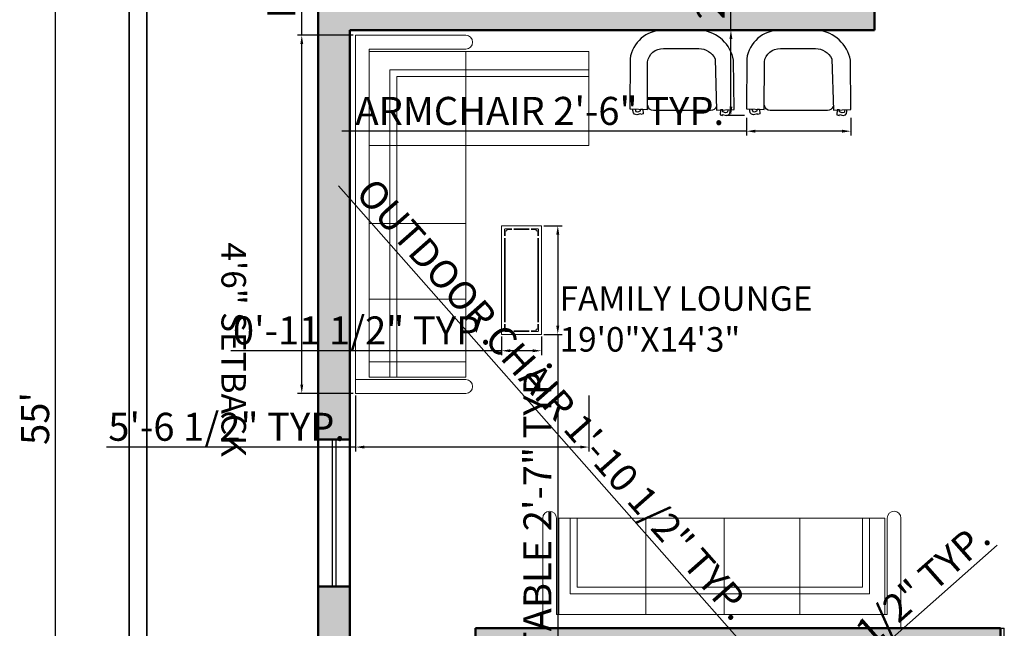
# Model space of a CAD drawing. Units: inches. Extents: x 3008 to 4088, y 1255 to 2137.
# Tile 25 of 30: x 3572 to 3853, y 1620 to 1794. Entities that reach past the tile are written whole.
import ezdxf

# ---------------------------------------------------------------- set-up
doc = ezdxf.new("R2010")
doc.units = ezdxf.units.IN
doc.layers.add('2D', color=7, linetype='Continuous')
for name, color, linetype, lineweight in [('A-ANNO-DIMS', 2, 'Continuous', 18), ('A-ANNO-TEXT', 7, 'Continuous', 18), ('A-AREA-IDEN', 7, 'Continuous', 18), ('A-DOOR', 4, 'Continuous', 25), ('A-FURN', 8, 'Continuous', 18), ('A-GLAZ', 4, 'Continuous', 25), ('A-WALL', 7, 'Continuous', 50), ('A-WALL-PATT', 8, 'Continuous', 13), ('C-PROP', 1, 'Continuous', 35)]:
    doc.layers.add(name, color=color, linetype=linetype, lineweight=lineweight)
doc.styles.get("Standard").update_dxf_attribs({"font": 'arial.ttf'})
doc.dimstyles.new('ISO-25', dxfattribs={"dimtxt": 8, "dimasz": 2.5, "dimexe": 1.25, "dimexo": 0.625, "dimtad": 1, "dimdec": 1, "dimlunit": 3, "dimtxsty": 'Standard', "dimcen": 2.5, "dimadec": 0, "dimazin": 0, "dimtfac": 1, "dimtdec": 1, "dimtmove": 0, "dimatfit": 3, "dimfxl": 1, "dimarcsym": 0})

# ---------------------------------------------------------------- blocks, each defined once
blk = doc.blocks.new('*D32')
at = {"layer": 'A-ANNO-DIMS', "color": 0, "lineweight": -2, "transparency": 16777216}
for p, q in [((3602.32, 2009.72), (3580.54, 2009.72)), ((3581.79, 2007.22), (3581.79, 1352.22)), ((3602.32, 1349.72), (3580.54, 1349.72))]:
    blk.add_line(p, q, dxfattribs=at)
at = {"layer": 'A-ANNO-DIMS', "color": 0, "transparency": 16777216}
for points in [[(3581.37, 2007.22), (3582.2, 2007.22), (3581.79, 2009.72)], [(3581.37, 1352.22), (3582.2, 1352.22), (3581.79, 1349.72)]]:
    blk.add_solid(points, dxfattribs=at)
at = {"layer": 'Defpoints', "color": 0, "transparency": 16777216}
for p in [(3602.94, 2009.72), (3581.79, 1349.72), (3602.94, 1349.72)]:
    blk.add_point(p, dxfattribs=at)
at = {"layer": 'A-ANNO-DIMS', "color": 0, "transparency": 16777216, "insert": (3577.09, 1679.72), "char_height": 8, "attachment_point": 5, "rotation": 90}
blk.add_mtext("55'", dxfattribs=at)
blk = doc.blocks.new('D1')
for p, q in [((1805.96, 1500.36), (1805.96, 1464.36)), ((1806.96, 1500.36), (1806.96, 1464.36)), ((1805.96, 1464.36), (1806.96, 1464.36))]:
    blk.add_line(p, q)
blk.add_arc((1805.96, 1464.36), 36, 0, 90)
blk = doc.blocks.new('S 1')
at = {"layer": '2D'}
blk.add_lwpolyline([(4300.17, 1811.07), (4294.36, 1811.27), (4294.5, 1827.76, -0.326306), (4305.18, 1837.77), (4318.07, 1837.77, -0.372891), (4329.09, 1828.23), (4329.16, 1811.54), (4323.28, 1811.34), (4323.21, 1827.16, 0.399039), (4317.87, 1831.63), (4306.12, 1831.63, 0.288471), (4300.71, 1828.23)], format="xyb", close=True, dxfattribs=at)
for points in [[(4296.37, 1811.14), (4296.63, 1810.34), (4297.23, 1810.21), (4298.1, 1810.54), (4298.1, 1811.14), (4298.9, 1811.14), (4299.04, 1809.54), (4298.24, 1809.34), (4298.17, 1809.61), (4296.9, 1809.27), (4296.17, 1809.47), (4295.77, 1809.94), (4295.63, 1810.74), (4295.63, 1811.21)], [(4327.35, 1811.41), (4327.09, 1810.61), (4326.49, 1810.47), (4325.62, 1810.81), (4325.62, 1811.41), (4324.82, 1811.41), (4324.68, 1809.81), (4325.48, 1809.61), (4325.55, 1809.87), (4326.82, 1809.54), (4327.55, 1809.74), (4327.95, 1810.21), (4328.09, 1811.01), (4328.09, 1811.47)]]:
    blk.add_lwpolyline(points, dxfattribs=at)
blk.add_lwpolyline([(4300.24, 1812.34, 0.33845), (4302.18, 1810.94), (4321.28, 1810.94, 0.381322), (4323.15, 1812.61, -0.892406)], format="xyb", dxfattribs=at)
blk = doc.blocks.new('TABLE-30A')
at = {"color": 0, "linetype": 'ByBlock'}
for p, q in [((0, 0), (0, 0.55)), ((0, 0.55), (1.5, 0.55)), ((1.5, 0.55), (1.5, 0)), ((0.051, 0.508), (0.042, 0.499)), ((0.042, 0.499), (0.042, 0.478)), ((0.042, 0.478), (0.072, 0.478)), ((0.042, 0.478), (0.042, 0.41)), ((0.072, 0.508), (0.051, 0.508)), ((0.051, 0.478), (0.051, 0.41)), ((0.072, 0.478), (0.072, 0.508)), ((0.072, 0.508), (0.14, 0.508)), ((0.072, 0.499), (0.14, 0.499)), ((1.331, 0.508), (0.169, 0.508)), ((1.331, 0.499), (0.169, 0.499)), ((1.428, 0.508), (1.36, 0.508)), ((1.428, 0.499), (1.36, 0.499)), ((1.428, 0.508), (1.428, 0.478)), ((1.449, 0.508), (1.428, 0.508)), ((1.428, 0.478), (1.458, 0.478)), ((1.458, 0.499), (1.449, 0.508)), ((1.449, 0.478), (1.449, 0.41)), ((1.458, 0.478), (1.458, 0.499)), ((1.458, 0.478), (1.458, 0.41)), ((0.042, 0.169), (0.042, 0.381)), ((0.051, 0.169), (0.051, 0.381)), ((1.449, 0.381), (1.449, 0.169)), ((1.458, 0.381), (1.458, 0.169)), ((0.042, 0.072), (0.042, 0.14)), ((0.051, 0.072), (0.051, 0.14)), ((1.449, 0.072), (1.449, 0.14)), ((1.458, 0.072), (1.458, 0.14)), ((1.5, 0), (0, 0)), ((0.042, 0.072), (0.042, 0.051)), ((0.072, 0.072), (0.042, 0.072)), ((0.042, 0.051), (0.051, 0.042)), ((0.051, 0.042), (0.072, 0.042)), ((0.072, 0.042), (0.072, 0.072)), ((0.072, 0.051), (0.14, 0.051)), ((0.072, 0.042), (0.14, 0.042)), ((0.169, 0.051), (1.331, 0.051)), ((0.169, 0.042), (1.331, 0.042)), ((1.428, 0.051), (1.36, 0.051)), ((1.428, 0.042), (1.36, 0.042)), ((1.428, 0.072), (1.428, 0.042)), ((1.458, 0.072), (1.428, 0.072)), ((1.428, 0.042), (1.449, 0.042)), ((1.449, 0.042), (1.458, 0.051)), ((1.458, 0.051), (1.458, 0.072))]:
    blk.add_line(p, q, dxfattribs=at)
blk = doc.blocks.new('SOFA-L')
for p, q in [((35.53, 102.74), (67.02, 102.74)), ((67.02, 102.74), (67.02, 0.37)), ((35.53, 98.8), (63.09, 98.8)), ((63.09, 98.8), (63.09, 4.97)), ((0.3, 98.14), (0.3, 71.24)), ((63.09, 98.14), (0.3, 98.14)), ((35.53, 4.97), (35.53, 98.14)), ((0.3, 92.9), (57.18, 92.9)), ((57.18, 92.9), (57.18, 4.97)), ((0.3, 90.93), (55.21, 90.93)), ((55.21, 90.93), (55.21, 4.97)), ((63.09, 71.24), (0.3, 71.24)), ((40.78, 71.24), (0.3, 71.24)), ((63.09, 48.93), (35.53, 48.93)), ((63.09, 27.28), (35.53, 27.28)), ((63.09, 9.36), (35.53, 9.36)), ((63.09, 4.97), (35.53, 4.97)), ((67.02, 4.31), (35.53, 4.31)), ((67.02, 0.37), (35.53, 0.37))]:
    blk.add_line(p, q)
for centre in [(35.53, 100.77), (35.53, 2.34)]:
    blk.add_arc(centre, 1.97, 90, 270)
blk = doc.blocks.new('*D51')
at = {"layer": 'A-ANNO-DIMS', "color": 0, "lineweight": -2, "transparency": 16777216}
for p, q in [((3778.81, 1614.68), (3662.79, 1746.22)), ((3776.72, 1612.84), (3779.74, 1615.51)), ((3792.2, 1599.5), (3780.46, 1612.81)), ((3791.76, 1595.78), (3794.79, 1598.45))]:
    blk.add_line(p, q, dxfattribs=at)
at = {"layer": 'A-ANNO-DIMS', "color": 0, "transparency": 16777216}
for points in [[(3780.77, 1613.08), (3780.15, 1612.53), (3778.81, 1614.68)], [(3792.51, 1599.77), (3791.89, 1599.22), (3793.85, 1597.62)]]:
    blk.add_solid(points, dxfattribs=at)
at = {"layer": 'Defpoints', "color": 0, "transparency": 16777216}
for p in [(3776.25, 1612.42), (3778.81, 1614.68), (3791.29, 1595.36)]:
    blk.add_point(p, dxfattribs=at)
at = {"layer": 'A-ANNO-DIMS', "color": 0, "transparency": 16777216, "insert": (3723.54, 1684.54), "char_height": 8, "attachment_point": 5, "rotation": 311.4119}
blk.add_mtext('OUTDOOR CHAIR 1\'-10 1/2" TYP.', dxfattribs=at)
blk = doc.blocks.new('*D52')
at = {"layer": 'A-ANNO-DIMS', "color": 0, "lineweight": -2, "transparency": 16777216}
for p, q in [((3793.55, 1592.8), (3851.01, 1643.48)), ((3791.71, 1594.89), (3794.38, 1591.87)), ((3778.59, 1579.61), (3791.68, 1591.15)), ((3774.87, 1580.05), (3777.54, 1577.02))]:
    blk.add_line(p, q, dxfattribs=at)
at = {"layer": 'A-ANNO-DIMS', "color": 0, "transparency": 16777216}
for points in [[(3791.4, 1591.46), (3791.95, 1590.84), (3793.55, 1592.8)], [(3778.32, 1579.92), (3778.87, 1579.3), (3776.72, 1577.96)]]:
    blk.add_solid(points, dxfattribs=at)
at = {"layer": 'Defpoints', "color": 0, "transparency": 16777216}
for p in [(3791.29, 1595.36), (3793.55, 1592.8), (3774.46, 1580.52)]:
    blk.add_point(p, dxfattribs=at)
at = {"layer": 'A-ANNO-DIMS', "color": 0, "transparency": 16777216, "insert": (3820.07, 1622.54), "char_height": 8, "attachment_point": 5, "rotation": 41.4119}
blk.add_mtext('1\'-10 1/2" TYP.', dxfattribs=at)
blk = doc.blocks.new('*D53')
at = {"layer": 'A-ANNO-DIMS', "color": 0, "lineweight": -2, "transparency": 16777216}
for p, q in [((3779.35, 1765.69), (3779.35, 1760.59)), ((3809.15, 1765.69), (3809.15, 1760.59)), ((3779.35, 1761.84), (3663.66, 1761.84)), ((3806.65, 1761.84), (3781.85, 1761.84))]:
    blk.add_line(p, q, dxfattribs=at)
at = {"layer": 'A-ANNO-DIMS', "color": 0, "transparency": 16777216}
for points in [[(3781.85, 1762.26), (3781.85, 1761.43), (3779.35, 1761.84)], [(3806.65, 1762.26), (3806.65, 1761.43), (3809.15, 1761.84)]]:
    blk.add_solid(points, dxfattribs=at)
at = {"layer": 'Defpoints', "color": 0, "transparency": 16777216}
for p in [(3779.35, 1766.31), (3809.15, 1766.31), (3779.35, 1761.84)]:
    blk.add_point(p, dxfattribs=at)
at = {"layer": 'A-ANNO-DIMS', "color": 0, "transparency": 16777216, "insert": (3720.26, 1766.61), "char_height": 8, "attachment_point": 5}
blk.add_mtext('ARMCHAIR 2\'-6" TYP.', dxfattribs=at)
blk = doc.blocks.new('*D54')
at = {"layer": 'A-ANNO-DIMS', "color": 0, "lineweight": -2, "transparency": 16777216}
for p, q in [((3774.89, 1790.72), (3774.89, 1862.01)), ((3778.73, 1790.72), (3773.64, 1790.72)), ((3774.89, 1768.81), (3774.89, 1788.22)), ((3778.73, 1766.31), (3773.64, 1766.31))]:
    blk.add_line(p, q, dxfattribs=at)
at = {"layer": 'A-ANNO-DIMS', "color": 0, "transparency": 16777216}
for points in [[(3774.47, 1788.22), (3775.3, 1788.22), (3774.89, 1790.72)], [(3774.47, 1768.81), (3775.3, 1768.81), (3774.89, 1766.31)]]:
    blk.add_solid(points, dxfattribs=at)
at = {"layer": 'Defpoints', "color": 0, "transparency": 16777216}
for p in [(3774.89, 1790.72), (3779.35, 1790.72), (3779.35, 1766.31)]:
    blk.add_point(p, dxfattribs=at)
at = {"layer": 'A-ANNO-DIMS', "color": 0, "transparency": 16777216, "insert": (3770.12, 1827.62), "char_height": 8, "attachment_point": 5, "rotation": 90}
blk.add_mtext('2\'-0 1/2" TYP.', dxfattribs=at)
blk = doc.blocks.new('*D55')
at = {"layer": 'A-ANNO-DIMS', "color": 0, "lineweight": -2, "transparency": 16777216}
for p, q in [((3721.38, 1734.8), (3726.66, 1734.8)), ((3725.41, 1732.3), (3725.41, 1706.23)), ((3721.38, 1703.73), (3726.66, 1703.73)), ((3725.41, 1703.73), (3725.41, 1563.75))]:
    blk.add_line(p, q, dxfattribs=at)
at = {"layer": 'A-ANNO-DIMS', "color": 0, "transparency": 16777216}
for points in [[(3724.99, 1732.3), (3725.83, 1732.3), (3725.41, 1734.8)], [(3724.99, 1706.23), (3725.83, 1706.23), (3725.41, 1703.73)]]:
    blk.add_solid(points, dxfattribs=at)
at = {"layer": 'Defpoints', "color": 0, "transparency": 16777216}
for p in [(3720.75, 1734.8), (3720.75, 1703.73), (3725.41, 1703.73)]:
    blk.add_point(p, dxfattribs=at)
at = {"layer": 'A-ANNO-DIMS', "color": 0, "transparency": 16777216, "insert": (3720.65, 1632.49), "char_height": 8, "attachment_point": 5, "rotation": 90}
blk.add_mtext('CENTRE TABLE 2\'-7" TYP.', dxfattribs=at)
blk = doc.blocks.new('*D56')
at = {"layer": 'A-ANNO-DIMS', "color": 0, "lineweight": -2, "transparency": 16777216}
for p, q in [((3709.36, 1703.11), (3709.36, 1697.82)), ((3720.75, 1703.11), (3720.75, 1697.82)), ((3709.36, 1699.07), (3631.99, 1699.07)), ((3718.25, 1699.07), (3711.86, 1699.07))]:
    blk.add_line(p, q, dxfattribs=at)
at = {"layer": 'A-ANNO-DIMS', "color": 0, "transparency": 16777216}
for points in [[(3711.86, 1699.49), (3711.86, 1698.66), (3709.36, 1699.07)], [(3718.25, 1699.49), (3718.25, 1698.66), (3720.75, 1699.07)]]:
    blk.add_solid(points, dxfattribs=at)
at = {"layer": 'Defpoints', "color": 0, "transparency": 16777216}
for p in [(3709.36, 1703.73), (3720.75, 1703.73), (3709.36, 1699.07)]:
    blk.add_point(p, dxfattribs=at)
at = {"layer": 'A-ANNO-DIMS', "color": 0, "transparency": 16777216, "insert": (3669.43, 1703.84), "char_height": 8, "attachment_point": 5}
blk.add_mtext('0\'-11 1/2" TYP.', dxfattribs=at)
blk = doc.blocks.new('*D57')
at = {"layer": 'A-ANNO-DIMS', "color": 0, "lineweight": -2, "transparency": 16777216}
for p, q in [((3652.25, 1789.25), (3652.25, 1903.53)), ((3666.98, 1789.25), (3651, 1789.25)), ((3652.25, 1689.39), (3652.25, 1786.75)), ((3666.98, 1686.89), (3651, 1686.89))]:
    blk.add_line(p, q, dxfattribs=at)
at = {"layer": 'A-ANNO-DIMS', "color": 0, "transparency": 16777216}
for points in [[(3651.83, 1786.75), (3652.67, 1786.75), (3652.25, 1789.25)], [(3651.83, 1689.39), (3652.67, 1689.39), (3652.25, 1686.89)]]:
    blk.add_solid(points, dxfattribs=at)
at = {"layer": 'Defpoints', "color": 0, "transparency": 16777216}
for p in [(3652.25, 1789.25), (3667.61, 1789.25), (3667.61, 1686.89)]:
    blk.add_point(p, dxfattribs=at)
at = {"layer": 'A-ANNO-DIMS', "color": 0, "transparency": 16777216, "insert": (3647.49, 1847.64), "char_height": 8, "attachment_point": 5, "rotation": 90}
blk.add_mtext('L-SOFA 8\'-6 1/2" TYP.', dxfattribs=at)
blk = doc.blocks.new('*D58')
at = {"layer": 'A-ANNO-DIMS', "color": 0, "lineweight": -2, "transparency": 16777216}
for p, q in [((3667.61, 1686.27), (3667.61, 1670.29)), ((3734.33, 1686.27), (3734.33, 1670.29)), ((3667.61, 1671.54), (3596.45, 1671.54)), ((3731.83, 1671.54), (3670.11, 1671.54))]:
    blk.add_line(p, q, dxfattribs=at)
at = {"layer": 'A-ANNO-DIMS', "color": 0, "transparency": 16777216}
for points in [[(3670.11, 1671.95), (3670.11, 1671.12), (3667.61, 1671.54)], [(3731.83, 1671.95), (3731.83, 1671.12), (3734.33, 1671.54)]]:
    blk.add_solid(points, dxfattribs=at)
at = {"layer": 'Defpoints', "color": 0, "transparency": 16777216}
for p in [(3667.61, 1686.89), (3734.33, 1686.89), (3667.61, 1671.54)]:
    blk.add_point(p, dxfattribs=at)
at = {"layer": 'A-ANNO-DIMS', "color": 0, "transparency": 16777216, "insert": (3630.78, 1676.3), "char_height": 8, "attachment_point": 5}
blk.add_mtext('5\'-6 1/2" TYP.', dxfattribs=at)

msp = doc.modelspace()

# ---------------------------------------------------------------- hatches: boundary and pattern name
at = {"layer": 'A-WALL-PATT'}
h = msp.add_hatch(color=256, dxfattribs=at)
h.dxf.hatch_style = 1
h.paths.add_polyline_path([(3665.94, 1631.72), (3656.94, 1631.72), (3656.94, 1546.72), (3665.94, 1546.72)])
h.paths.add_polyline_path([(3851.94, 1619.72), (3701.94, 1619.72), (3701.94, 1610.72), (3788.94, 1610.72), (3788.94, 1469.72), (3809.94, 1469.72), (3809.94, 1478.72), (3797.94, 1478.72), (3797.94, 1550.72), (3815.94, 1550.72), (3815.94, 1556.72), (3797.94, 1556.72), (3797.94, 1610.72), (3845.94, 1610.72), (3845.94, 1586.72), (3851.94, 1586.72)])
h.paths.add_polyline_path([(4028.94, 1631.72), (4019.94, 1631.72), (4019.94, 1619.72), (3887.94, 1619.72), (3887.94, 1610.72), (4019.94, 1610.72), (4019.94, 1577.72), (4028.94, 1577.72)])
h.paths.add_polyline_path([(3875.94, 1478.72), (3851.94, 1478.72), (3851.94, 1556.72), (3845.94, 1556.72), (3845.94, 1526.72), (3845.94, 1478.72), (3833.94, 1478.72), (3833.94, 1469.72), (3875.94, 1469.72)])
h.paths.add_polyline_path([(3959.94, 1478.72), (3917.94, 1478.72), (3917.94, 1469.72), (3959.94, 1469.72)])
h.paths.add_polyline_path([(4028.94, 1511.72), (4019.94, 1511.72), (4019.94, 1478.72), (4001.94, 1478.72), (4001.94, 1469.72), (4028.94, 1469.72)])
h.paths.add_polyline_path([(4028.94, 1699.22), (4019.94, 1699.22), (4019.94, 1673.72), (3893.94, 1673.72), (3893.94, 1649.72), (3899.94, 1649.72), (3899.94, 1667.72), (4019.94, 1667.72), (4019.94, 1655.72), (4028.94, 1655.72)])
h.paths.add_polyline_path([(4028.94, 1847.72), (4019.94, 1847.72), (4019.94, 1796.72), (3863.94, 1796.72), (3863.94, 1790.72), (4019.94, 1790.72), (4019.94, 1765.22), (4028.94, 1765.22)])
h.paths.add_polyline_path([(3815.94, 1796.72), (3779.94, 1796.72), (3665.94, 1796.72), (3665.94, 1898.72), (3656.94, 1898.72), (3656.94, 1673.72), (3665.94, 1673.72), (3665.94, 1790.72), (3815.94, 1790.72)])
h.paths.add_polyline_path([(3755.94, 1949.72), (3656.94, 1949.72), (3656.94, 1940.72), (3665.94, 1940.72), (3755.94, 1940.72)])
h.paths.add_polyline_path([(3827.94, 1949.72), (3797.94, 1949.72), (3797.94, 1940.72), (3809.94, 1940.72), (3809.94, 1874.72), (3815.94, 1874.72), (3815.94, 1940.72), (3827.94, 1940.72)])
h.paths.add_polyline_path([(3953.94, 1949.72), (3851.94, 1949.72), (3851.94, 1940.72), (3863.94, 1940.72), (3863.94, 1844.72), (3809.94, 1844.72), (3809.94, 1832.72), (3815.94, 1832.72), (3815.94, 1838.72), (3863.94, 1838.72), (3869.94, 1838.72), (3869.94, 1940.72), (3953.94, 1940.72)])
h.paths.add_polyline_path([(4028.94, 1949.72), (3995.94, 1949.72), (3995.94, 1940.72), (4019.94, 1940.72), (4019.94, 1889.72), (4028.94, 1889.72)])

# ---------------------------------------------------------------- linework, layer by layer
at = {"layer": 'A-FURN'}
for p, q in [((3721.12, 1651.22), (3721.12, 1619.72)), ((3725.05, 1651.22), (3725.05, 1623.66)), ((3818.89, 1651.22), (3725.71, 1651.22)), ((3725.71, 1623.66), (3725.71, 1651.22)), ((3728.96, 1651.22), (3728.96, 1629.56)), ((3730.93, 1651.22), (3730.93, 1631.53)), ((3750.61, 1623.66), (3750.61, 1651.22)), ((3750.61, 1645.97), (3750.61, 1651.22)), ((3772.92, 1623.66), (3772.92, 1651.22)), ((3794.58, 1623.66), (3794.58, 1651.22)), ((3812.49, 1631.53), (3812.49, 1651.22)), ((3814.49, 1629.56), (3814.49, 1651.22)), ((3818.89, 1623.66), (3818.89, 1651.22)), ((3819.54, 1623.66), (3819.54, 1651.22)), ((3823.48, 1619.72), (3823.48, 1651.22)), ((3728.96, 1629.56), (3814.49, 1629.56)), ((3730.93, 1631.53), (3812.49, 1631.53)), ((3725.05, 1623.66), (3819.54, 1623.66)), ((3721.12, 1619.72), (3823.48, 1619.72))]:
    msp.add_line(p, q, dxfattribs=at)
for centre in [(3723.08, 1651.22), (3821.51, 1651.22)]:
    msp.add_arc(centre, 1.97, 0, 180, dxfattribs=at)
at = {"layer": 'A-GLAZ'}
for p, q in [((3660.94, 1673.72), (3660.94, 1631.72)), ((3660.94, 1673.72), (3660.94, 1631.72)), ((3661.94, 1673.72), (3661.94, 1631.72))]:
    msp.add_line(p, q, dxfattribs=at)
at = {"layer": 'A-WALL'}
for p, q in [((3656.94, 1546.72), (3656.94, 1949.72)), ((3815.94, 1790.72), (3815.94, 1796.72)), ((3665.94, 1790.72), (3815.94, 1790.72)), ((3665.94, 1546.72), (3665.94, 1790.72)), ((3656.94, 1673.72), (3665.94, 1673.72)), ((3656.94, 1631.72), (3665.94, 1631.72)), ((3701.94, 1619.72), (3851.94, 1619.72)), ((3701.94, 1610.72), (3701.94, 1619.72)), ((3851.94, 1586.72), (3851.94, 1619.72))]:
    msp.add_line(p, q, dxfattribs=at)
at = {"layer": 'C-PROP'}
for p, q in [((3602.94, 1349.72), (3602.94, 2009.72)), ((3607.94, 1354.72), (3607.94, 2004.72))]:
    msp.add_line(p, q, dxfattribs=at)

# ---------------------------------------------------------------- block references
at = {"layer": 'A-DOOR', "xscale": -1, "rotation": 180}
msp.add_blockref('D1', (2045.98, 3084.08), dxfattribs=at)
at = {"layer": 'A-FURN', "xscale": -0.8563117011609614, "yscale": 0.8563117011609614, "zscale": 0.8563117011609614}
for p in [(7453.1, 217.01), (7486.46, 217.01)]:
    msp.add_blockref('S 1', p, dxfattribs=at)
at = {"layer": 'A-FURN', "extrusion": (0, 0, -1), "zscale": -1}
msp.add_blockref('SOFA-L', (-3734.63, 1686.52), dxfattribs=at)
at = {"layer": 'A-FURN', "xscale": -20.70834898381633, "yscale": 20.70834898381633, "zscale": 20.70834898381633, "rotation": 90}
msp.add_blockref('TABLE-30A', (3720.75, 1734.8), dxfattribs=at)

# ---------------------------------------------------------------- texts
at = {"layer": 'A-ANNO-TEXT', "insert": (3636.3, 1730.05), "char_height": 7, "attachment_point": 1, "rotation": 270}
msp.add_mtext_dynamic_manual_height_columns('{\\fTimes New Roman|b0|i0|c0|p18;4\'6" SETBACK}', width=105.6127, gutter_width=12.5, heights=[0], dxfattribs=at)
at = {"layer": 'A-AREA-IDEN', "insert": (3725.92, 1717.5), "char_height": 7, "attachment_point": 1}
msp.add_mtext_dynamic_manual_height_columns('{\\fTimes New Roman|b0|i0|c0|p18;FAMILY LOUNGE    19\'0"X14\'3"}', width=105.6127, gutter_width=12.5, heights=[0], dxfattribs=at)

# ---------------------------------------------------------------- dimensions: what is measured, and where the dimension line sits
at = {"layer": 'A-ANNO-DIMS'}
dim = msp.add_linear_dim(base=(3581.79, 1349.72), p1=(3602.94, 2009.72), p2=(3602.94, 1349.72), angle=90, dimstyle='ISO-25', override={"dimclrd": 0, "dimclre": 0, "dimclrt": 0}, dxfattribs=at)
dim.commit()
dim.dimension.update_dxf_attribs({"geometry": '*D32', "text_midpoint": (3577.09, 1679.72)})
for base, p1, p2, angle, text, picture, middle in [((3652.25, 1789.25), (3667.61, 1686.89), (3667.61, 1789.25), 90, 'L-SOFA <> TYP.', '*D57', (3647.49, 1847.64)), ((3774.89, 1790.72), (3779.35, 1766.31), (3779.35, 1790.72), 90, '<> TYP.', '*D54', (3770.12, 1827.62)), ((3779.35, 1761.84), (3809.15, 1766.31), (3779.35, 1766.31), 180, 'ARMCHAIR <> TYP.', '*D53', (3720.26, 1766.61)), ((3778.81, 1614.68), (3791.29, 1595.36), (3776.25, 1612.42), 131.4119, 'OUTDOOR CHAIR <> TYP.', '*D51', (3723.54, 1684.54)), ((3725.41, 1703.73), (3720.75, 1734.8), (3720.75, 1703.73), 270, 'CENTRE TABLE <> TYP.', '*D55', (3720.65, 1632.49)), ((3709.36, 1699.07), (3720.75, 1703.73), (3709.36, 1703.73), 180, '<> TYP.', '*D56', (3669.43, 1703.84)), ((3667.61, 1671.54), (3734.33, 1686.89), (3667.61, 1686.89), 180, '<> TYP.', '*D58', (3630.78, 1676.3)), ((3793.55, 1592.8), (3774.46, 1580.52), (3791.29, 1595.36), 41.4119, '<> TYP.', '*D52', (3820.07, 1622.54))]:
    dim = msp.add_linear_dim(base=base, p1=p1, p2=p2, angle=angle, text=text, dimstyle='ISO-25', override={"dimdec": 1, "dimrnd": 0, "dimzin": 1, "dimlunit": 4, "dimfrac": 2}, dxfattribs=at)
    dim.commit()
    dim.dimension.update_dxf_attribs({"geometry": picture, "text_midpoint": middle})

doc.saveas('drawing.dxf')
